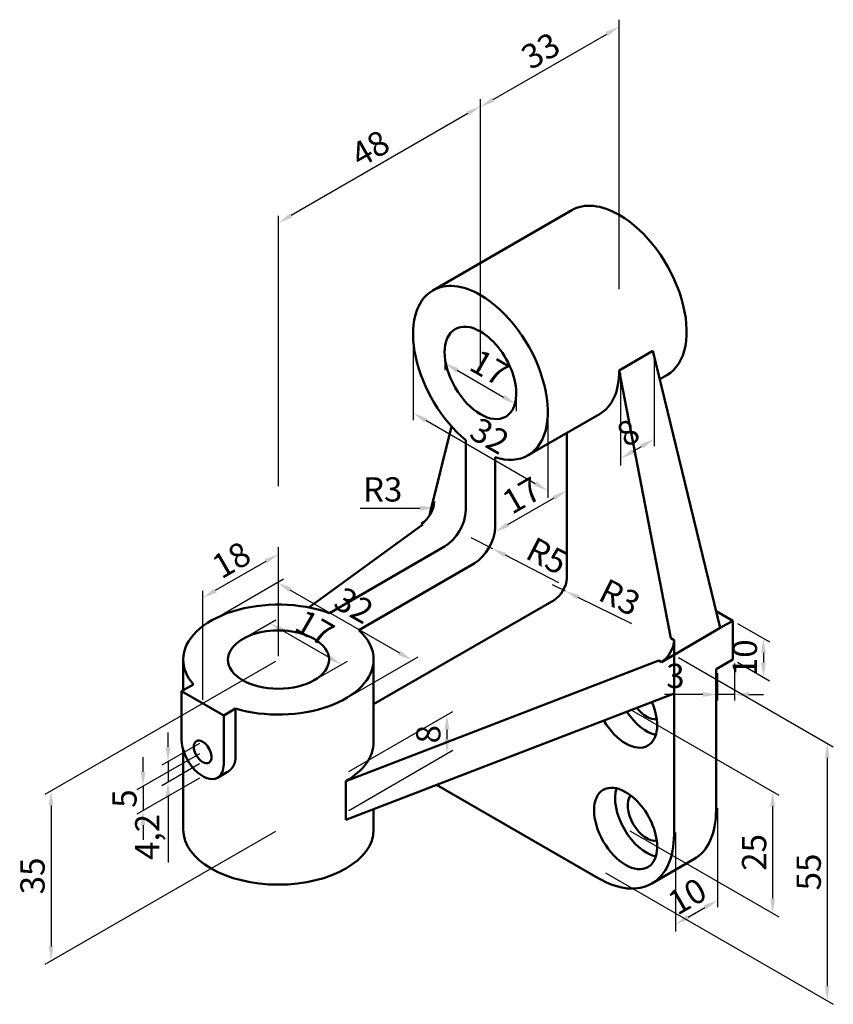
# Model space of a CAD drawing. Units: millimetres. Extents: x 259 to 427, y 185 to 388.
import ezdxf

# ---------------------------------------------------------------- set-up
doc = ezdxf.new("R2010")
doc.units = ezdxf.units.MM
doc.layers.add('M-DIMS', color=2, linetype='Continuous', lineweight=25)
doc.layers.add('M-OUTL', color=7, linetype='Continuous', lineweight=50)
doc.styles.get("Standard").update_dxf_attribs({"font": 'arial.ttf'})
doc.dimstyles.new('ISO-25', dxfattribs={"dimtxt": 5, "dimasz": 3, "dimexe": 1.25, "dimexo": 0.625, "dimtad": 1, "dimtxsty": 'Standard', "dimcen": 2.5, "dimadec": 0, "dimazin": 0, "dimtfac": 1, "dimtmove": 0, "dimatfit": 3, "dimfxl": 1, "dimarcsym": 0})

# ---------------------------------------------------------------- blocks, each defined once
blk = doc.blocks.new('*D1')
at = {"layer": 'Defpoints', "color": 0, "transparency": 16777216}
for p in [(406.19, 264.03), (406.19, 256.03), (412.18, 252.58)]:
    blk.add_point(p, dxfattribs=at)
at = {"layer": 'M-DIMS', "color": 0, "lineweight": -2, "transparency": 16777216}
for p, q in [((406.82, 263.67), (413.43, 259.86)), ((412.18, 257.58), (412.18, 255.58)), ((406.82, 255.67), (413.43, 251.86))]:
    blk.add_line(p, q, dxfattribs=at)
at = {"layer": 'M-DIMS', "color": 0, "transparency": 16777216}
for points in [[(411.68, 257.58), (412.68, 257.58), (412.18, 260.58)], [(411.68, 255.58), (412.68, 255.58), (412.18, 252.58)]]:
    blk.add_solid(points, dxfattribs=at)
at = {"layer": 'M-DIMS', "color": 0, "transparency": 16777216, "insert": (409, 256.58), "char_height": 5, "attachment_point": 5, "rotation": 90}
blk.add_mtext('10', dxfattribs=at)
blk = doc.blocks.new('*D2')
at = {"layer": 'Defpoints', "color": 0, "transparency": 16777216}
for p in [(406.19, 256.03), (402.73, 254.03), (402.73, 249.03)]:
    blk.add_point(p, dxfattribs=at)
at = {"layer": 'M-DIMS', "color": 0, "lineweight": -2, "transparency": 16777216}
for p, q in [((406.19, 255.41), (406.19, 247.78)), ((402.73, 253.41), (402.73, 247.78)), ((399.73, 249.03), (391.81, 249.03)), ((406.19, 249.03), (402.73, 249.03)), ((409.19, 249.03), (412.19, 249.03))]:
    blk.add_line(p, q, dxfattribs=at)
at = {"layer": 'M-DIMS', "color": 0, "transparency": 16777216}
for points in [[(399.73, 249.53), (399.73, 248.53), (402.73, 249.03)], [(409.19, 249.53), (409.19, 248.53), (406.19, 249.03)]]:
    blk.add_solid(points, dxfattribs=at)
at = {"layer": 'M-DIMS', "color": 0, "transparency": 16777216, "insert": (394.07, 252.21), "char_height": 5, "attachment_point": 5}
blk.add_mtext('3', dxfattribs=at)
blk = doc.blocks.new('*D3')
at = {"layer": 'Defpoints', "color": 0, "transparency": 16777216}
for p in [(394.07, 257.03), (379.07, 212.69), (425.31, 186)]:
    blk.add_point(p, dxfattribs=at)
at = {"layer": 'M-DIMS', "color": 0, "lineweight": -2, "transparency": 16777216}
for p, q in [((394.69, 256.67), (426.56, 238.28)), ((425.31, 236), (425.31, 189)), ((379.69, 212.33), (426.56, 185.28))]:
    blk.add_line(p, q, dxfattribs=at)
at = {"layer": 'M-DIMS', "color": 0, "transparency": 16777216}
for points in [[(424.81, 236), (425.81, 236), (425.31, 239)], [(424.81, 189), (425.81, 189), (425.31, 186)]]:
    blk.add_solid(points, dxfattribs=at)
at = {"layer": 'M-DIMS', "color": 0, "transparency": 16777216, "insert": (422.14, 212.5), "char_height": 5, "attachment_point": 5, "rotation": 90}
blk.add_mtext('55', dxfattribs=at)
blk = doc.blocks.new('*D4')
at = {"layer": 'Defpoints', "color": 0, "transparency": 16777216}
for p in [(384.07, 246.35), (414.08, 229.03), (384.07, 221.35)]:
    blk.add_point(p, dxfattribs=at)
at = {"layer": 'M-DIMS', "color": 0, "lineweight": -2, "transparency": 16777216}
for p, q in [((384.69, 245.99), (415.33, 228.3)), ((414.08, 207.03), (414.08, 226.03)), ((384.69, 220.99), (415.33, 203.3))]:
    blk.add_line(p, q, dxfattribs=at)
at = {"layer": 'M-DIMS', "color": 0, "transparency": 16777216}
for points in [[(413.58, 226.03), (414.58, 226.03), (414.08, 229.03)], [(413.58, 207.03), (414.58, 207.03), (414.08, 204.03)]]:
    blk.add_solid(points, dxfattribs=at)
at = {"layer": 'M-DIMS', "color": 0, "transparency": 16777216, "insert": (410.91, 216.53), "char_height": 5, "attachment_point": 5, "rotation": 90}
blk.add_mtext('25', dxfattribs=at)
blk = doc.blocks.new('*D5')
at = {"layer": 'Defpoints', "color": 0, "transparency": 16777216}
for p in [(389.72, 319.86), (382.79, 315.86), (389.72, 301.59)]:
    blk.add_point(p, dxfattribs=at)
at = {"layer": 'M-DIMS', "color": 0, "lineweight": -2, "transparency": 16777216}
for p, q in [((389.72, 319.14), (389.72, 300.15)), ((382.79, 315.14), (382.79, 296.15)), ((385.39, 299.09), (387.12, 300.09))]:
    blk.add_line(p, q, dxfattribs=at)
at = {"layer": 'M-DIMS', "color": 0, "transparency": 16777216}
for points in [[(386.87, 300.52), (387.37, 299.66), (389.72, 301.59)], [(385.14, 299.52), (385.64, 298.66), (382.79, 297.59)]]:
    blk.add_solid(points, dxfattribs=at)
at = {"layer": 'M-DIMS', "color": 0, "transparency": 16777216, "insert": (384.66, 302.34), "char_height": 5, "attachment_point": 5, "rotation": 30}
blk.add_mtext('8', dxfattribs=at)
blk = doc.blocks.new('*D6')
at = {"layer": 'Defpoints', "color": 0, "transparency": 16777216}
for p in [(347.04, 236.85), (326.22, 232.82), (326.22, 224.83)]:
    blk.add_point(p, dxfattribs=at)
at = {"layer": 'M-DIMS', "color": 0, "lineweight": -2, "transparency": 16777216}
for p, q in [((326.85, 233.18), (348.29, 245.56)), ((347.04, 241.84), (347.04, 239.85)), ((326.85, 225.19), (348.29, 237.57))]:
    blk.add_line(p, q, dxfattribs=at)
at = {"layer": 'M-DIMS', "color": 0, "transparency": 16777216}
for points in [[(346.54, 241.84), (347.54, 241.84), (347.04, 244.84)], [(346.54, 239.85), (347.54, 239.85), (347.04, 236.85)]]:
    blk.add_solid(points, dxfattribs=at)
at = {"layer": 'M-DIMS', "color": 0, "transparency": 16777216, "insert": (343.86, 240.85), "char_height": 5, "attachment_point": 5, "rotation": 90}
blk.add_mtext('8', dxfattribs=at)
blk = doc.blocks.new('*D7')
at = {"layer": 'Defpoints', "color": 0, "transparency": 16777216}
for p in [(312.37, 256.2), (312.37, 221.2), (265.58, 194.19)]:
    blk.add_point(p, dxfattribs=at)
at = {"layer": 'M-DIMS', "color": 0, "lineweight": -2, "transparency": 16777216}
for p, q in [((311.74, 255.84), (264.33, 228.47)), ((265.58, 226.19), (265.58, 197.19)), ((311.74, 220.84), (264.33, 193.47))]:
    blk.add_line(p, q, dxfattribs=at)
at = {"layer": 'M-DIMS', "color": 0, "transparency": 16777216}
for points in [[(265.08, 226.19), (266.08, 226.19), (265.58, 229.19)], [(265.08, 197.19), (266.08, 197.19), (265.58, 194.19)]]:
    blk.add_solid(points, dxfattribs=at)
at = {"layer": 'M-DIMS', "color": 0, "transparency": 16777216, "insert": (262.41, 211.69), "char_height": 5, "attachment_point": 5, "rotation": 90}
blk.add_mtext('35', dxfattribs=at)
blk = doc.blocks.new('*D8')
at = {"layer": 'Defpoints', "color": 0, "transparency": 16777216}
for p in [(296.78, 268.91), (312.37, 256.2), (296.78, 247.2)]:
    blk.add_point(p, dxfattribs=at)
at = {"layer": 'M-DIMS', "color": 0, "lineweight": -2, "transparency": 16777216}
for p, q in [((312.37, 256.93), (312.37, 279.35)), ((309.77, 276.41), (299.38, 270.41)), ((296.78, 247.93), (296.78, 270.35))]:
    blk.add_line(p, q, dxfattribs=at)
at = {"layer": 'M-DIMS', "color": 0, "transparency": 16777216}
for points in [[(309.52, 276.84), (310.02, 275.97), (312.37, 277.91)], [(299.13, 270.84), (299.63, 269.97), (296.78, 268.91)]]:
    blk.add_solid(points, dxfattribs=at)
at = {"layer": 'M-DIMS', "color": 0, "transparency": 16777216, "insert": (302.99, 276.16), "char_height": 5, "attachment_point": 5, "rotation": 30}
blk.add_mtext('18', dxfattribs=at)
blk = doc.blocks.new('*D9')
at = {"layer": 'Defpoints', "color": 0, "transparency": 16777216}
for p in [(296.78, 237.2), (296.78, 232.2), (284.5, 225.11)]:
    blk.add_point(p, dxfattribs=at)
at = {"layer": 'M-DIMS', "color": 0, "lineweight": -2, "transparency": 16777216}
for p, q in [((296.16, 236.84), (283.25, 229.39)), ((284.5, 233.11), (284.5, 236.11)), ((296.16, 231.84), (283.25, 224.39)), ((284.5, 230.11), (284.5, 225.11)), ((284.5, 222.11), (284.5, 219.11))]:
    blk.add_line(p, q, dxfattribs=at)
at = {"layer": 'M-DIMS', "color": 0, "transparency": 16777216}
for points in [[(284, 233.11), (285, 233.11), (284.5, 230.11)], [(284, 222.11), (285, 222.11), (284.5, 225.11)]]:
    blk.add_solid(points, dxfattribs=at)
at = {"layer": 'M-DIMS', "color": 0, "transparency": 16777216, "insert": (281.33, 227.61), "char_height": 5, "attachment_point": 5, "rotation": 90}
blk.add_mtext('5', dxfattribs=at)
blk = doc.blocks.new('*D10')
at = {"layer": 'Defpoints', "color": 0, "transparency": 16777216}
for p in [(296.78, 239.3), (296.78, 235.1), (289.65, 230.98)]:
    blk.add_point(p, dxfattribs=at)
at = {"layer": 'M-DIMS', "color": 0, "lineweight": -2, "transparency": 16777216}
for p, q in [((289.65, 238.18), (289.65, 241.18)), ((296.16, 238.94), (288.4, 234.46)), ((289.65, 235.18), (289.65, 230.98)), ((296.16, 234.74), (288.4, 230.26)), ((289.65, 227.98), (289.65, 214.48))]:
    blk.add_line(p, q, dxfattribs=at)
at = {"layer": 'M-DIMS', "color": 0, "transparency": 16777216}
for points in [[(289.15, 238.18), (290.15, 238.18), (289.65, 235.18)], [(289.15, 227.98), (290.15, 227.98), (289.65, 230.98)]]:
    blk.add_solid(points, dxfattribs=at)
at = {"layer": 'M-DIMS', "color": 0, "transparency": 16777216, "insert": (286.02, 219.73), "char_height": 5, "attachment_point": 5, "rotation": 90}
blk.add_mtext('4,2', dxfattribs=at)
blk = doc.blocks.new('*D11')
at = {"layer": 'Defpoints', "color": 0, "transparency": 16777216}
for p in [(305.01, 260.45), (325.34, 255.19), (319.73, 251.95)]:
    blk.add_point(p, dxfattribs=at)
at = {"layer": 'M-DIMS', "color": 0, "lineweight": -2, "transparency": 16777216}
for p, q in [((305.63, 260.81), (311.86, 264.41)), ((313.21, 262.19), (322.74, 256.69)), ((320.35, 252.31), (326.59, 255.91))]:
    blk.add_line(p, q, dxfattribs=at)
at = {"layer": 'M-DIMS', "color": 0, "transparency": 16777216}
for points in [[(313.46, 262.62), (312.96, 261.76), (310.61, 263.69)], [(322.99, 257.12), (322.49, 256.26), (325.34, 255.19)]]:
    blk.add_solid(points, dxfattribs=at)
at = {"layer": 'M-DIMS', "color": 0, "transparency": 16777216, "insert": (319.54, 262.16), "char_height": 5, "attachment_point": 5, "rotation": 330}
blk.add_mtext('17', dxfattribs=at)
blk = doc.blocks.new('*D12')
at = {"layer": 'Defpoints', "color": 0, "transparency": 16777216}
for p in [(298.51, 264.2), (339.86, 256.08), (326.22, 248.2)]:
    blk.add_point(p, dxfattribs=at)
at = {"layer": 'M-DIMS', "color": 0, "lineweight": -2, "transparency": 16777216}
for p, q in [((299.14, 264.56), (313.4, 272.8)), ((314.75, 270.58), (337.27, 257.58)), ((326.85, 248.56), (341.11, 256.8))]:
    blk.add_line(p, q, dxfattribs=at)
at = {"layer": 'M-DIMS', "color": 0, "transparency": 16777216}
for points in [[(315, 271.01), (314.5, 270.15), (312.15, 272.08)], [(337.52, 258.01), (337.02, 257.15), (339.86, 256.08)]]:
    blk.add_solid(points, dxfattribs=at)
at = {"layer": 'M-DIMS', "color": 0, "transparency": 16777216, "insert": (327.6, 266.83), "char_height": 5, "attachment_point": 5, "rotation": 330}
blk.add_mtext('32', dxfattribs=at)
blk = doc.blocks.new('*D13')
at = {"layer": 'Defpoints', "color": 0, "transparency": 16777216}
for p in [(341.48, 287.4), (344.48, 287.4)]:
    blk.add_point(p, dxfattribs=at)
at = {"layer": 'M-DIMS', "color": 0, "lineweight": -2, "transparency": 16777216}
blk.add_line((329.17, 287.4), (341.48, 287.4), dxfattribs=at)
at = {"layer": 'M-DIMS', "color": 0, "transparency": 16777216}
blk.add_solid([(341.48, 287.9), (341.48, 286.9), (344.48, 287.4)], dxfattribs=at)
at = {"layer": 'M-DIMS', "color": 0, "transparency": 16777216, "insert": (333.82, 290.58), "char_height": 5, "attachment_point": 5}
blk.add_mtext('R3', dxfattribs=at)
blk = doc.blocks.new('*D14')
at = {"layer": 'Defpoints', "color": 0, "transparency": 16777216}
for p in [(351.97, 281.34), (356.41, 279.05)]:
    blk.add_point(p, dxfattribs=at)
at = {"layer": 'M-DIMS', "color": 0, "lineweight": -2, "transparency": 16777216}
for p, q in [((351.97, 281.34), (356.41, 279.05)), ((370.06, 272.03), (359.08, 277.68))]:
    blk.add_line(p, q, dxfattribs=at)
at = {"layer": 'M-DIMS', "color": 0, "transparency": 16777216}
blk.add_solid([(359.31, 278.12), (358.85, 277.24), (356.41, 279.05)], dxfattribs=at)
at = {"layer": 'M-DIMS', "color": 0, "transparency": 16777216, "insert": (367.36, 276.98), "char_height": 5, "attachment_point": 5, "rotation": 332.7656}
blk.add_mtext('R5', dxfattribs=at)
blk = doc.blocks.new('*D15')
at = {"layer": 'Defpoints', "color": 0, "transparency": 16777216}
for p in [(368.69, 271.69), (371.38, 270.35)]:
    blk.add_point(p, dxfattribs=at)
at = {"layer": 'M-DIMS', "color": 0, "lineweight": -2, "transparency": 16777216}
for p, q in [((368.69, 271.69), (371.38, 270.35)), ((385.09, 263.54), (374.06, 269.02))]:
    blk.add_line(p, q, dxfattribs=at)
at = {"layer": 'M-DIMS', "color": 0, "transparency": 16777216}
blk.add_solid([(374.29, 269.46), (373.84, 268.57), (371.38, 270.35)], dxfattribs=at)
at = {"layer": 'M-DIMS', "color": 0, "transparency": 16777216, "insert": (382.34, 268.46), "char_height": 5, "attachment_point": 5, "rotation": 333.5741}
blk.add_mtext('R3', dxfattribs=at)
blk = doc.blocks.new('*D16')
at = {"layer": 'Defpoints', "color": 0, "transparency": 16777216}
for p in [(371.69, 290.98), (371.69, 289.84), (356.97, 281.34)]:
    blk.add_point(p, dxfattribs=at)
at = {"layer": 'M-DIMS', "color": 0, "lineweight": -2, "transparency": 16777216}
for p, q in [((371.69, 290.56), (371.69, 292.43)), ((359.57, 283.98), (369.09, 289.48)), ((356.97, 282.06), (356.97, 283.93))]:
    blk.add_line(p, q, dxfattribs=at)
at = {"layer": 'M-DIMS', "color": 0, "transparency": 16777216}
for points in [[(368.84, 289.92), (369.34, 289.05), (371.69, 290.98)], [(359.32, 284.42), (359.82, 283.55), (356.97, 282.48)]]:
    blk.add_solid(points, dxfattribs=at)
at = {"layer": 'M-DIMS', "color": 0, "transparency": 16777216, "insert": (362.76, 289.45), "char_height": 5, "attachment_point": 5, "rotation": 30}
blk.add_mtext('17', dxfattribs=at)
blk = doc.blocks.new('*D17')
at = {"layer": 'Defpoints', "color": 0, "transparency": 16777216}
for p in [(346.58, 319.45), (361.3, 310.95), (361.3, 308.74)]:
    blk.add_point(p, dxfattribs=at)
at = {"layer": 'M-DIMS', "color": 0, "lineweight": -2, "transparency": 16777216}
for p, q in [((346.58, 318.73), (346.58, 315.8)), ((349.17, 315.74), (358.7, 310.24)), ((361.3, 310.23), (361.3, 307.3))]:
    blk.add_line(p, q, dxfattribs=at)
at = {"layer": 'M-DIMS', "color": 0, "transparency": 16777216}
for points in [[(349.42, 316.17), (348.92, 315.31), (346.58, 317.24)], [(358.95, 310.67), (358.45, 309.81), (361.3, 308.74)]]:
    blk.add_solid(points, dxfattribs=at)
at = {"layer": 'M-DIMS', "color": 0, "transparency": 16777216, "insert": (355.51, 315.71), "char_height": 5, "attachment_point": 5, "rotation": 330}
blk.add_mtext('17', dxfattribs=at)
blk = doc.blocks.new('*D18')
at = {"layer": 'Defpoints', "color": 0, "transparency": 16777216}
for p in [(340.08, 323.2), (367.79, 307.2), (367.79, 290.95)]:
    blk.add_point(p, dxfattribs=at)
at = {"layer": 'M-DIMS', "color": 0, "lineweight": -2, "transparency": 16777216}
for p, q in [((340.08, 322.48), (340.08, 305.5)), ((367.79, 306.48), (367.79, 289.5)), ((342.68, 305.45), (365.2, 292.45))]:
    blk.add_line(p, q, dxfattribs=at)
at = {"layer": 'M-DIMS', "color": 0, "transparency": 16777216}
for points in [[(342.93, 305.88), (342.43, 305.01), (340.08, 306.95)], [(365.45, 292.88), (364.95, 292.01), (367.79, 290.95)]]:
    blk.add_solid(points, dxfattribs=at)
at = {"layer": 'M-DIMS', "color": 0, "transparency": 16777216, "insert": (355.53, 301.7), "char_height": 5, "attachment_point": 5, "rotation": 330}
blk.add_mtext('32', dxfattribs=at)
blk = doc.blocks.new('*D19')
at = {"layer": 'Defpoints', "color": 0, "transparency": 16777216}
for p in [(312.37, 346.08), (353.94, 315.2), (312.37, 291.2)]:
    blk.add_point(p, dxfattribs=at)
at = {"layer": 'M-DIMS', "color": 0, "lineweight": -2, "transparency": 16777216}
for p, q in [((353.94, 315.93), (353.94, 371.52)), ((351.34, 368.58), (314.97, 347.58)), ((312.37, 291.93), (312.37, 347.52))]:
    blk.add_line(p, q, dxfattribs=at)
at = {"layer": 'M-DIMS', "color": 0, "transparency": 16777216}
for points in [[(351.09, 369.01), (351.59, 368.15), (353.94, 370.08)], [(314.72, 348.01), (315.22, 347.15), (312.37, 346.08)]]:
    blk.add_solid(points, dxfattribs=at)
at = {"layer": 'M-DIMS', "color": 0, "transparency": 16777216, "insert": (331.56, 360.83), "char_height": 5, "attachment_point": 5, "rotation": 30}
blk.add_mtext('48', dxfattribs=at)
blk = doc.blocks.new('*D20')
at = {"layer": 'Defpoints', "color": 0, "transparency": 16777216}
for p in [(382.52, 386.44), (382.52, 331.7), (353.94, 315.2)]:
    blk.add_point(p, dxfattribs=at)
at = {"layer": 'M-DIMS', "color": 0, "lineweight": -2, "transparency": 16777216}
for p, q in [((382.52, 332.43), (382.52, 387.89)), ((356.54, 371.44), (379.92, 384.94)), ((353.94, 315.93), (353.94, 371.39))]:
    blk.add_line(p, q, dxfattribs=at)
at = {"layer": 'M-DIMS', "color": 0, "transparency": 16777216}
for points in [[(379.67, 385.38), (380.17, 384.51), (382.52, 386.44)], [(356.29, 371.88), (356.79, 371.01), (353.94, 369.94)]]:
    blk.add_solid(points, dxfattribs=at)
at = {"layer": 'M-DIMS', "color": 0, "transparency": 16777216, "insert": (366.64, 380.95), "char_height": 5, "attachment_point": 5, "rotation": 30}
blk.add_mtext('33', dxfattribs=at)
blk = doc.blocks.new('*D21')
at = {"layer": 'Defpoints', "color": 0, "transparency": 16777216}
for p in [(402.73, 226.35), (394.07, 221.35), (402.73, 206.69)]:
    blk.add_point(p, dxfattribs=at)
at = {"layer": 'M-DIMS', "color": 0, "lineweight": -2, "transparency": 16777216}
for p, q in [((402.73, 225.63), (402.73, 205.25)), ((394.07, 220.63), (394.07, 200.25)), ((396.67, 203.19), (400.13, 205.19))]:
    blk.add_line(p, q, dxfattribs=at)
at = {"layer": 'M-DIMS', "color": 0, "transparency": 16777216}
for points in [[(399.88, 205.63), (400.38, 204.76), (402.73, 206.69)], [(396.42, 203.63), (396.92, 202.76), (394.07, 201.69)]]:
    blk.add_solid(points, dxfattribs=at)
at = {"layer": 'M-DIMS', "color": 0, "transparency": 16777216, "insert": (396.81, 206.95), "char_height": 5, "attachment_point": 5, "rotation": 30}
blk.add_mtext('10', dxfattribs=at)

msp = doc.modelspace()

# ---------------------------------------------------------------- linework, layer by layer
at = {"layer": 'M-OUTL'}
for p, q in [((344.14, 332.185), (372.719, 348.685)), ((382.517, 315.714), (389.445, 319.714)), ((389.445, 319.714), (403.301, 262.714)), ((393.125, 260.589), (382.517, 315.714)), ((390.858, 313.903), (392.315, 314.744)), ((363.736, 298.244), (378.458, 306.744)), ((347.994, 304.193), (343.545, 286.214)), ((371.691, 272.964), (371.691, 302.837)), ((350.907, 286.964), (350.907, 301.352)), ((356.969, 283.464), (356.969, 297.852)), ((343.545, 285.978), (343.545, 286.214)), ((342.113, 284.041), (318.618, 266.937)), ((342.113, 284.041), (341.813, 284.214)), ((322.858, 265.771), (346.577, 279.464)), ((328.92, 262.271), (352.639, 275.964)), ((331.964, 247.028), (369.093, 268.464)), ((405.899, 264.214), (402.453, 266.204)), ((403.301, 262.714), (405.899, 264.214)), ((405.899, 256.214), (405.899, 264.214)), ((393.775, 257.214), (403.301, 262.714)), ((393.775, 260.214), (393.125, 260.589)), ((393.775, 257.214), (393.775, 260.214)), ((292.773, 249.901), (292.773, 256.214)), ((326.225, 231.214), (390.657, 256.014)), ((331.964, 239.214), (331.964, 256.214)), ((391.177, 255.714), (390.657, 256.014)), ((391.177, 255.714), (393.775, 257.214)), ((393.775, 249.214), (393.775, 257.214)), ((402.435, 254.214), (405.899, 256.214)), ((402.435, 225.214), (402.435, 254.214)), ((292.45, 249.714), (294.876, 251.115)), ((301.11, 244.714), (292.45, 249.714)), ((292.45, 239.714), (292.45, 249.714)), ((326.225, 223.214), (393.775, 249.214)), ((393.775, 220.214), (393.775, 249.214)), ((301.11, 244.714), (303.536, 246.115)), ((303.536, 236.115), (303.536, 246.115)), ((301.11, 234.714), (301.11, 244.714)), ((292.773, 221.214), (292.773, 237.634)), ((299.842, 231.911), (301.917, 233.109)), ((326.225, 223.214), (326.225, 231.214)), ((378.187, 211.214), (344.931, 230.414)), ((331.964, 221.214), (331.964, 225.423)), ((389.209, 210.122), (397.869, 215.122))]:
    msp.add_line(p, q, dxfattribs=at)
msp.add_lwpolyline([(303.536, 236.115), (303.536, 236.076), (303.536, 236.037), (303.535, 235.997), (303.533, 235.959), (303.532, 235.92), (303.53, 235.881), (303.528, 235.842), (303.525, 235.804), (303.522, 235.766), (303.518, 235.727), (303.515, 235.689), (303.511, 235.651), (303.506, 235.613), (303.501, 235.576), (303.496, 235.538), (303.491, 235.5), (303.485, 235.463), (303.479, 235.426), (303.472, 235.389), (303.465, 235.352), (303.458, 235.315), (303.45, 235.278), (303.442, 235.242), (303.434, 235.205), (303.425, 235.169), (303.416, 235.133), (303.407, 235.097), (303.397, 235.061), (303.387, 235.025), (303.376, 234.99), (303.366, 234.954), (303.354, 234.919), (303.343, 234.884), (303.331, 234.849), (303.319, 234.814), (303.306, 234.78), (303.293, 234.745), (303.28, 234.711), (303.266, 234.677), (303.252, 234.643), (303.238, 234.61), (303.223, 234.576), (303.208, 234.543), (303.193, 234.51), (303.177, 234.477), (303.161, 234.444), (303.145, 234.411), (303.128, 234.379), (303.111, 234.347), (303.093, 234.315), (303.075, 234.283), (303.057, 234.251), (303.039, 234.22), (303.02, 234.189), (303.001, 234.158), (302.981, 234.127), (302.961, 234.096), (302.941, 234.066), (302.92, 234.036), (302.899, 234.006), (302.878, 233.977), (302.856, 233.947), (302.834, 233.918), (302.812, 233.889), (302.789, 233.86), (302.766, 233.832), (302.743, 233.804), (302.719, 233.776), (302.695, 233.748), (302.671, 233.721), (302.646, 233.693), (302.621, 233.666), (302.596, 233.64), (302.57, 233.613), (302.544, 233.587), (302.517, 233.561), (302.49, 233.536), (302.463, 233.511), (302.436, 233.486), (302.408, 233.461), (302.38, 233.437), (302.351, 233.412), (302.322, 233.389), (302.293, 233.365), (302.264, 233.342), (302.234, 233.319), (302.204, 233.297), (302.173, 233.274), (302.142, 233.252), (302.111, 233.231), (302.079, 233.21), (302.047, 233.189), (302.015, 233.168), (301.983, 233.148), (301.95, 233.128), (301.917, 233.109)], dxfattribs=at)
for centre, major_axis, start_param, end_param in [((382.517, 331.714), (9.798, -16.971), 2.3561945, 3.1415927), ((382.517, 331.714), (9.798, -16.971), 0, 2.3561945), ((353.938, 315.214), (9.798, -16.971), 2.3561945, 3.1415927), ((353.938, 315.214), (9.798, -16.971), 3.1415927, 5.2772539), ((353.938, 315.214), (9.798, -16.971), 0, 2.3561945), ((353.938, 315.214), (5.205, -9.016), 3.1415927, 6.2831853), ((353.938, 315.214), (5.205, -9.016), 2.3561945, 3.1415927), ((353.938, 315.214), (5.205, -9.016), 0, 2.3561945), ((368.66, 323.714), (9.798, -16.971), 0, 0.7853982), ((353.938, 315.214), (9.798, -16.971), 5.7183204, 6.2831853), ((341.813, 287.214), (1.837, 3.182), 3.927014, 5.497764), ((346.576, 284.464), (3.062, 5.303), 3.927014, 5.497764), ((352.639, 280.964), (3.062, 5.303), 3.927014, 5.497764), ((369.093, 271.464), (-1.837, -3.182), 0.7854213, 2.3561713), ((312.369, 256.214), (19.596, 0), 1.0059314, 3.1415927), ((312.369, 256.214), (10.41, 0), 0.7853982, 3.1415927), ((312.369, 256.214), (19.596, 0), 0, 0.5648649), ((312.369, 256.214), (10.41, 0), 0, 0.7853982), ((391.177, 258.714), (1.837, 3.182), 3.927014, 5.497764), ((312.369, 256.214), (19.596, 0), 3.1415927, 3.6091671), ((312.369, 256.214), (10.41, 0), 3.1415927, 6.2831853), ((312.369, 256.214), (19.596, 0), 4.2448145, 6.2831853), ((383.816, 246.464), (4.593, -7.955), 0, 1.3689421), ((388.146, 248.964), (4.593, -7.955), 4.8193358, 5.7923026), ((388.146, 248.964), (2.756, -4.773), 4.9550737, 6.0613823), ((383.816, 246.464), (4.593, -7.955), 4.7329234, 6.2831853), ((296.78, 237.214), (3.062, -5.303), 3.9269908, 6.2831853), ((296.78, 237.214), (1.286, -2.227), 3.1415927, 6.2831853), ((296.78, 237.214), (1.286, -2.227), 2.3561945, 3.1415927), ((296.78, 237.214), (1.286, -2.227), 0, 2.3561945), ((312.369, 239.214), (19.596, 0), 5.4977871, 6.2831853), ((296.78, 237.214), (3.062, -5.303), 0, 0.7853982), ((383.816, 221.464), (4.593, -7.955), 3.1415927, 6.2831853), ((383.816, 221.464), (4.593, -7.955), 2.3561945, 3.1415927), ((388.146, 223.964), (4.593, -7.955), 3.6324753, 5.7923026), ((383.816, 221.464), (4.593, -7.955), 0, 2.3561945), ((388.146, 223.964), (2.756, -4.773), 3.3633956, 6.0613823), ((386.847, 234.214), (11.023, -19.092), 0, 0.7853982), ((312.369, 221.214), (19.596, 0), 3.1415927, 6.2831853), ((378.187, 229.214), (11.023, -19.092), 0, 0.7853982), ((378.187, 229.214), (11.023, -19.092), 5.4977871, 6.2831853)]:
    msp.add_ellipse(centre, major_axis=major_axis, ratio=0.5773503, start_param=start_param, end_param=end_param, dxfattribs=at)

# ---------------------------------------------------------------- dimensions: what is measured, and where the dimension line sits
at = {"layer": 'M-DIMS'}
for p1, p2, distance, picture, middle in [((353.938, 315.204), (382.517, 331.704), 47.405, '*D20', (366.637, 380.947)), ((353.938, 315.204), (312.369, 291.204), -47.525, '*D19', (331.564, 360.833)), ((340.081, 323.204), (367.794, 307.204), -14.079, '*D18', (355.528, 301.701)), ((346.577, 319.454), (361.299, 310.954), -1.917, '*D17', (355.505, 315.705)), ((382.788, 315.861), (389.717, 319.861), -15.823, '*D5', (384.663, 302.342)), ((356.969, 281.341), (371.691, 289.841), 0.989, '*D16', (362.762, 289.448)), ((312.369, 256.204), (296.78, 247.204), -18.794, '*D8', (302.985, 276.158)), ((298.512, 264.204), (326.225, 248.204), 13.639, '*D12', (327.597, 266.832)), ((305.007, 260.454), (319.73, 251.954), 5.606, '*D11', (319.542, 262.156)), ((394.069, 221.355), (402.729, 226.355), -17.027, '*D21', (396.81, 206.945))]:
    dim = msp.add_aligned_dim(p1=p1, p2=p2, distance=distance, dimstyle='ISO-25', override={"dimclrd": 0, "dimclre": 0, "dimclrt": 0}, dxfattribs=at)
    dim.commit()
    dim.dimension.update_dxf_attribs({"geometry": picture, "text_midpoint": middle})
dim = msp.add_radius_dim(center=(341.481, 287.396), mpoint=(344.481, 287.396), dimstyle='ISO-25', override={"dimclrd": 0, "dimclre": 0, "dimclrt": 0}, dxfattribs=at)
dim.commit()
dim.dimension.update_dxf_attribs({"geometry": '*D13', "text_midpoint": (333.825, 287.396), "dimtype": 164})
for center, mpoint, picture, middle in [((351.969, 281.341), (356.415, 279.053), '*D14', (367.356, 276.984)), ((368.691, 271.686), (371.378, 270.351), '*D15', (382.336, 268.456))]:
    dim = msp.add_radius_dim(center=center, mpoint=mpoint, dimstyle='ISO-25', override={"dimclrd": 0, "dimclre": 0, "dimclrt": 0}, dxfattribs=at)
    dim.commit()
    dim.dimension.update_dxf_attribs({"geometry": picture, "text_midpoint": middle})
for base, p1, p2, text, picture, middle in [((412.182, 252.577), (406.193, 264.034), (406.193, 256.034), '10', '*D1', (409.004, 256.577)), ((425.308, 185.998), (394.069, 257.034), (379.069, 212.695), '55', '*D3', (422.14, 212.498)), ((347.04, 236.851), (326.225, 232.823), (326.225, 224.833), '8', '*D6', (343.862, 240.846))]:
    dim = msp.add_linear_dim(base=base, p1=p1, p2=p2, angle=90, text=text, dimstyle='ISO-25', override={"dimclrd": 0, "dimclre": 0, "dimclrt": 0}, dxfattribs=at)
    dim.commit()
    dim.dimension.update_dxf_attribs({"geometry": picture, "text_midpoint": middle})
for base, p1, p2, picture, middle in [((265.585, 194.193), (312.369, 256.204), (312.369, 221.204), '*D7', (262.405, 211.693)), ((414.084, 229.025), (384.069, 221.355), (384.069, 246.355), '*D4', (410.906, 216.525)), ((289.645, 230.985), (296.78, 239.304), (296.78, 235.104), '*D10', (286.015, 219.733)), ((284.498, 225.113), (296.78, 237.204), (296.78, 232.204), '*D9', (281.331, 227.613))]:
    dim = msp.add_linear_dim(base=base, p1=p1, p2=p2, angle=90, dimstyle='ISO-25', override={"dimclrd": 0, "dimclre": 0, "dimclrt": 0}, dxfattribs=at)
    dim.commit()
    dim.dimension.update_dxf_attribs({"geometry": picture, "text_midpoint": middle})
dim = msp.add_linear_dim(base=(402.729, 249.034), p1=(406.193, 256.034), p2=(402.729, 254.034), text='3', dimstyle='ISO-25', override={"dimclrd": 0, "dimclre": 0, "dimclrt": 0}, dxfattribs=at)
dim.commit()
dim.dimension.update_dxf_attribs({"geometry": '*D2', "text_midpoint": (394.069, 249.034), "dimtype": 160})

doc.saveas('drawing.dxf')
